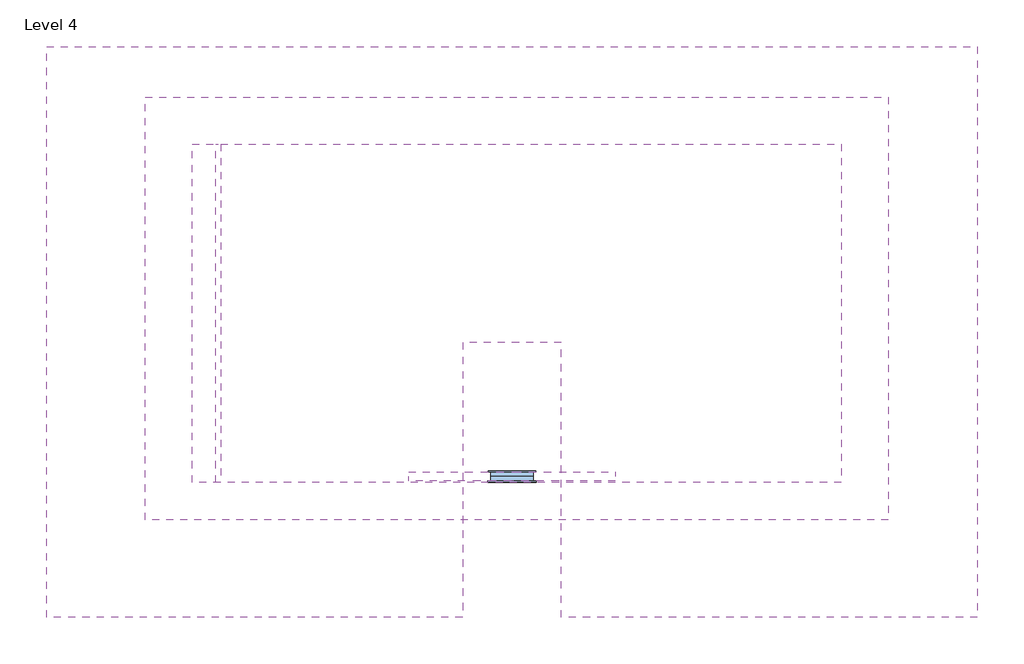
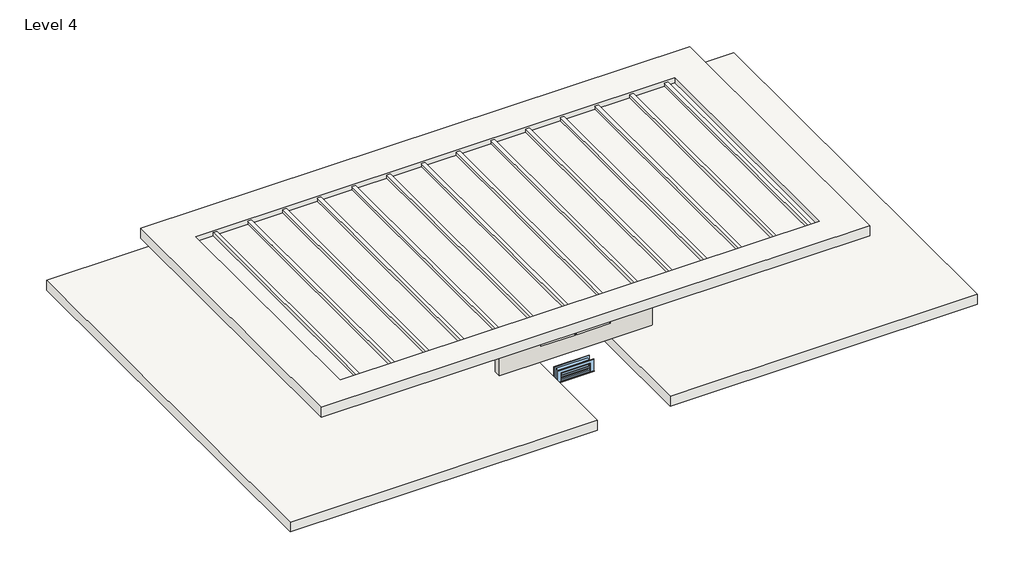
# One storey: 4 slabs, 1 wall, 1 window.
"""IFC4 building model written with IfcOpenShell, lengths in millimetres."""

from ifc_helpers import new_model, si_unit, frame, origin, place, context, project, spatial, polyline, outline, extrude, transform, mapped, element, save
from components import window_e4bd14ab

model = new_model("IFC4")

# Units and contexts
model_context = context("Model", 3, world=origin())
ifc_project = project(units=[si_unit("LENGTHUNIT", "METRE", prefix="MILLI")], contexts=[model_context])

# Site, building, storey
site = spatial("IfcSite", under=ifc_project)
building = spatial("IfcBuilding", under=site)
storey = spatial("IfcBuildingStorey", under=building, Name="Level 4", Elevation=9144.0)

# Slabs
placement = place(None, origin())
element("IfcSlab", 1, ObjectType="Generic - 12\"", at=placement, inside=storey, context=model_context, shape_type="SweptSolid", body=[
    extrude(outline(polyline([(2123.1661524, 12293.8223265), (2123.1661524, -50.5776735), (-6868.4338476, -50.5776735), (-6868.4338476, 5893.0223265), (-9002.0338476, 5893.0223265), (-9002.0338476, -50.5776735), (-17993.6338476, -50.5776735), (-17993.6338476, 12293.8223265), (2123.1661524, 12293.8223265)])), frame((0.0, 0.0, 10363.2), z_axis=(0.0, 0.0, 1.0), x_axis=(1.0, 0.0, 0.0)), (0.0, 0.0, 1.0), 304.8),
])
element("IfcSlab", 2, ObjectType="Generic - 12\"", at=placement, inside=storey, context=model_context, shape_type="SweptSolid", body=[
    extrude(outline(polyline([(-1128.0338476, 10185.6223265), (-1026.4338476, 10185.6223265), (-1026.4338476, 2870.4223265), (-1128.0338476, 2870.4223265), (-1128.0338476, 10185.6223265)])), frame((0.0, 0.0, 11836.4), z_axis=(0.0, 0.0, 1.0), x_axis=(1.0, 0.0, 0.0)), (0.0, 0.0, 1.0), 304.8),
    extrude(outline(polyline([(-2042.4338476, 2870.4223265), (-2144.0338476, 2870.4223265), (-2144.0338476, 10185.6223265), (-2042.4338476, 10185.6223265), (-2042.4338476, 2870.4223265)])), frame((0.0, 0.0, 11836.4), z_axis=(0.0, 0.0, 1.0), x_axis=(1.0, 0.0, 0.0)), (0.0, 0.0, 1.0), 304.8),
    extrude(outline(polyline([(-3058.4338476, 2870.4223265), (-3160.0338476, 2870.4223265), (-3160.0338476, 10185.6223265), (-3058.4338476, 10185.6223265), (-3058.4338476, 2870.4223265)])), frame((0.0, 0.0, 11836.4), z_axis=(0.0, 0.0, 1.0), x_axis=(1.0, 0.0, 0.0)), (0.0, 0.0, 1.0), 304.8),
    extrude(outline(polyline([(-4074.4338476, 2870.4223265), (-4176.0338476, 2870.4223265), (-4176.0338476, 10185.6223265), (-4074.4338476, 10185.6223265), (-4074.4338476, 2870.4223265)])), frame((0.0, 0.0, 11836.4), z_axis=(0.0, 0.0, 1.0), x_axis=(1.0, 0.0, 0.0)), (0.0, 0.0, 1.0), 304.8),
    extrude(outline(polyline([(-5090.4338476, 2870.4223265), (-5192.0338476, 2870.4223265), (-5192.0338476, 10185.6223265), (-5090.4338476, 10185.6223265), (-5090.4338476, 2870.4223265)])), frame((0.0, 0.0, 11836.4), z_axis=(0.0, 0.0, 1.0), x_axis=(1.0, 0.0, 0.0)), (0.0, 0.0, 1.0), 304.8),
    extrude(outline(polyline([(-6106.4338476, 2870.4223265), (-6208.0338476, 2870.4223265), (-6208.0338476, 10185.6223265), (-6106.4338476, 10185.6223265), (-6106.4338476, 2870.4223265)])), frame((0.0, 0.0, 11836.4), z_axis=(0.0, 0.0, 1.0), x_axis=(1.0, 0.0, 0.0)), (0.0, 0.0, 1.0), 304.8),
    extrude(outline(polyline([(-7122.4338476, 2870.4223265), (-7224.0338476, 2870.4223265), (-7224.0338476, 10185.6223265), (-7122.4338476, 10185.6223265), (-7122.4338476, 2870.4223265)])), frame((0.0, 0.0, 11836.4), z_axis=(0.0, 0.0, 1.0), x_axis=(1.0, 0.0, 0.0)), (0.0, 0.0, 1.0), 304.8),
    extrude(outline(polyline([(-8138.4338476, 2870.4223265), (-8240.0338476, 2870.4223265), (-8240.0338476, 10185.6223265), (-8138.4338476, 10185.6223265), (-8138.4338476, 2870.4223265)])), frame((0.0, 0.0, 11836.4), z_axis=(0.0, 0.0, 1.0), x_axis=(1.0, 0.0, 0.0)), (0.0, 0.0, 1.0), 304.8),
    extrude(outline(polyline([(-9154.4338476, 2870.4223265), (-9256.0338476, 2870.4223265), (-9256.0338476, 10185.6223265), (-9154.4338476, 10185.6223265), (-9154.4338476, 2870.4223265)])), frame((0.0, 0.0, 11836.4), z_axis=(0.0, 0.0, 1.0), x_axis=(1.0, 0.0, 0.0)), (0.0, 0.0, 1.0), 304.8),
    extrude(outline(polyline([(-10170.4338476, 2870.4223265), (-10272.0338476, 2870.4223265), (-10272.0338476, 10185.6223265), (-10170.4338476, 10185.6223265), (-10170.4338476, 2870.4223265)])), frame((0.0, 0.0, 11836.4), z_axis=(0.0, 0.0, 1.0), x_axis=(1.0, 0.0, 0.0)), (0.0, 0.0, 1.0), 304.8),
    extrude(outline(polyline([(-11186.4338476, 2870.4223265), (-11288.0338476, 2870.4223265), (-11288.0338476, 10185.6223265), (-11186.4338476, 10185.6223265), (-11186.4338476, 2870.4223265)])), frame((0.0, 0.0, 11836.4), z_axis=(0.0, 0.0, 1.0), x_axis=(1.0, 0.0, 0.0)), (0.0, 0.0, 1.0), 304.8),
    extrude(outline(polyline([(-12202.4338476, 2870.4223265), (-12304.0338476, 2870.4223265), (-12304.0338476, 10185.6223265), (-12202.4338476, 10185.6223265), (-12202.4338476, 2870.4223265)])), frame((0.0, 0.0, 11836.4), z_axis=(0.0, 0.0, 1.0), x_axis=(1.0, 0.0, 0.0)), (0.0, 0.0, 1.0), 304.8),
    extrude(outline(polyline([(-13218.4338476, 2870.4223265), (-13320.0338476, 2870.4223265), (-13320.0338476, 10185.6223265), (-13218.4338476, 10185.6223265), (-13218.4338476, 2870.4223265)])), frame((0.0, 0.0, 11836.4), z_axis=(0.0, 0.0, 1.0), x_axis=(1.0, 0.0, 0.0)), (0.0, 0.0, 1.0), 304.8),
    extrude(outline(polyline([(-14234.4338476, 2870.4223265), (-14336.0338476, 2870.4223265), (-14336.0338476, 10185.6223265), (-14234.4338476, 10185.6223265), (-14234.4338476, 2870.4223265)])), frame((0.0, 0.0, 11836.4), z_axis=(0.0, 0.0, 1.0), x_axis=(1.0, 0.0, 0.0)), (0.0, 0.0, 1.0), 304.8),
])
element("IfcSlab", 3, ObjectType="Generic - 12\"", at=placement, inside=storey, context=model_context, shape_type="SweptSolid", body=[
    extrude(outline(polyline([(192.7661524, 11201.6223265), (192.7661524, 2057.6223265), (-15860.0338476, 2057.6223265), (-15860.0338476, 11201.6223265), (192.7661524, 11201.6223265)]), holes=[polyline([(-823.2338476, 10185.6223265), (-14844.0338476, 10185.6223265), (-14844.0338476, 2870.4223265), (-823.2338476, 2870.4223265), (-823.2338476, 10185.6223265)])]), frame((0.0, 0.0, 11887.2), z_axis=(0.0, 0.0, 1.0), x_axis=(1.0, 0.0, 0.0)), (0.0, 0.0, 1.0), 304.8),
])
element("IfcSlab", 4, ObjectType="Generic - 6\"", at=placement, inside=storey, context=model_context, shape_type="SweptSolid", body=[
    extrude(outline(polyline([(-823.2338476, 2870.4223265), (-14844.0338476, 2870.4223265), (-14844.0338476, 10185.6223265), (-823.2338476, 10185.6223265), (-823.2338476, 2870.4223265)])), frame((0.0, 0.0, 11887.2), z_axis=(0.0, 0.0, 1.0), x_axis=(1.0, 0.0, 0.0)), (0.0, 0.0, 1.0), 152.4),
])

# Wall
element("IfcWall", 5, ObjectType="Generic - 8\"", at=placement, inside=storey, context=model_context, shape_type="SweptSolid", body=[
    extrude(outline(polyline([(10668.0, -5700.0338476), (11887.2, -5700.0338476), (11887.2, -10170.4338476), (10668.0, -10170.4338476), (10668.0, -5700.0338476)]), holes=[polyline([(11582.4, -6919.2338476), (11379.2, -6919.2338476), (11379.2, -7903.4838476), (11582.4, -7903.4838476), (11582.4, -6919.2338476)]), polyline([(11353.8, -7903.4838476), (11353.8, -6919.2338476), (11150.6, -6919.2338476), (11150.6, -7903.4838476), (11353.8, -7903.4838476)]), polyline([(11582.4, -8951.2338476), (11582.4, -7941.5838476), (11379.2, -7941.5838476), (11379.2, -8951.2338476), (11582.4, -8951.2338476)]), polyline([(11353.8, -8951.2338476), (11353.8, -7939.8332262), (11150.6, -7939.8332262), (11150.6, -8951.2338476), (11353.8, -8951.2338476)])]), frame((0.0, 2895.8223265, 0.0), z_axis=(0.0, 1.0, 0.0), x_axis=(0.0, 0.0, 1.0)), (0.0, 0.0, 1.0), 203.2),
])

# Window
window_shape = window_e4bd14ab(model_context)
element("IfcWindow", 6, ObjectType="Double Hung with Trim : 36\" x 12\"", at=placement, inside=storey, context=model_context, shape_type="MappedRepresentation", body=[
    mapped(window_shape, transform((-7935.2338476, 2997.4223265, 8937.4050177), x_axis=(-1.0, 0.0, 0.0), y_axis=(0.0, -1.0, 0.0), z_axis=(0.0, 0.0, 1.0))),
])

save(model, "model.ifc")

# Revit data of these elements
# Type "Generic - 12\""
#   Assembly Code = "B1010"
#   Function = 0
#   Layers, outside or top first: 1' - 0" "Concrete Masonry Units" (function 1)
# Type "Generic - 6\""
#   Assembly Code = "B1010"
#   Function = 0
#   Layers, outside or top first: 0' - 6" "Concrete, Precast" (function 1)
# Type "Generic - 8\""
#   Assembly Code = "B2010"
#   Layers, outside or top first: 0' - 8" no material (function 1)
# Type "Double Hung with Trim : 36\" x 12\""
#   Type Mark = "21"
#   Construction Type Id = "GSP4R"
#   Assembly Code = "B2020100"
#   Analytic Construction = "1/8 in Pilkington single glazing"
#   Visual Light Transmittance = 0.9
#   Solar Heat Gain Coefficient = 0.78
#   Heat Transfer Coefficient (U) = 0.6496 BTU/(h·ft²·°F)
#   Height = 1' - 0"
#   Default Sill Height = 3' - 0"
#   Trim Projection - Ext. = 0' - 0 1/2"
#   Trim Projection - Int. = 0' - 0 3/4"
#   Trim Width - Exterior = 0' - 3 1/2"
#   Trim Width - Interior = 0' - 3 1/2"
#   Width = 3' - 0"
#   Window Inset = 0' - 0 3/4"
#   Define Thermal Properties by = 1
#   Glass Pane Material = Glass
#   Sash Material = Iron, Ductile
#   Trim Exterior Material = Iron, Ductile
#   Trim Interior Material = Iron, Ductile
#   Wall Closure = (empty or 0)
# Element 1 (IfcSlab, "Generic - 12\"")
#   Height Offset From Level = 5' - 0"
#   Phase Created = New Construction
#   Materials on its faces: "Concrete Masonry Units"
# Element 2 (IfcSlab, "Generic - 12\"")
#   built-in parameter 1001955 = 3.14159 (stored number, unit not read)
#   Height Offset From Level = 9' - 10"
#   Phase Created = New Construction
#   Materials on its faces: "Concrete Masonry Units"
# Element 3 (IfcSlab, "Generic - 12\"")
#   Height Offset From Level = 10' - 0"
#   Phase Created = New Construction
#   Materials on its faces: "Concrete Masonry Units"
# Element 4 (IfcSlab, "Generic - 6\"")
#   Height Offset From Level = 9' - 6"
#   Phase Created = New Construction
#   Materials on its faces: "Concrete, Precast"
# Element 5 (IfcWall, "Generic - 8\"")
#   built-in parameter 1001111 = 5' - 0"
#   Top Offset = 0' - 0"
#   Base Offset = 5' - 0"
#   Unconnected Height = 4' - 0"
#   wall height = 4' - 0"
#   Phase Created = New Construction
#   Base Constraint = Level 4
#   Materials on its faces: "Default Wall"
# Element 6 (IfcWindow, "Double Hung with Trim : 36\" x 12\"")
#   Mark = "26"
#   Phase Created = New Construction
#   Materials on its faces: "Iron, Ductile", "Glass"
# Materials
#   "Concrete Masonry Units": class "Masonry", colour RGB 227 227 227, transparency 0, Description = "Concrete masonry units", Cost = 0
#   "Concrete, Precast": class "Concrete", colour RGB 198 187 187, transparency 0, Description = "Precast concrete", Cost = 0
#   "Glass": class "Glass", colour RGB 0 128 192, transparency 0.75, Description = "Soda Lime Glass", Cost = 0
#   "Iron, Ductile": class "Metal", colour RGB 0 0 0, transparency 0, Description = "Ductile cast iron", Cost = 0
#   "Default Wall": colour RGB 128 128 128, transparency 0
